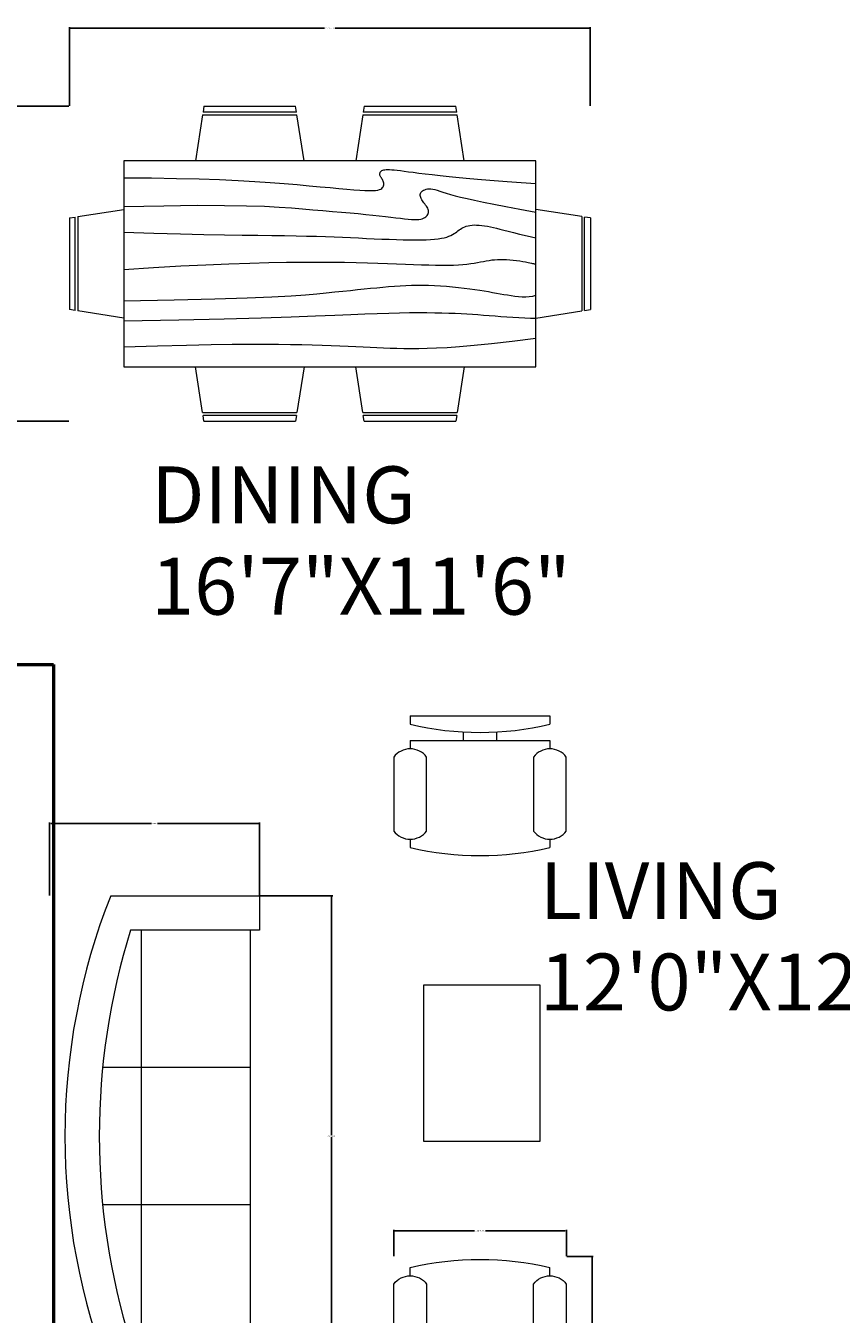
# Model space of a CAD drawing. Units: inches. Extents: x 614 to 1202, y 131 to 752.
# Tile 3 of 5: x 862 to 1005, y 293 to 518. Entities that reach past the tile are written whole.
import ezdxf

# ---------------------------------------------------------------- set-up
doc = ezdxf.new("R2010")
doc.units = ezdxf.units.IN
doc.header["$MEASUREMENT"] = 0
for name, color, linetype, lineweight in [('A-ANNO-DIMS', 2, 'Continuous', 18), ('A-AREA-IDEN', 7, 'Continuous', 18), ('A-FURN', 8, 'Continuous', 18), ('A-WALL', 7, 'Continuous', 50)]:
    doc.layers.add(name, color=color, linetype=linetype, lineweight=lineweight)
doc.styles.get("Standard").update_dxf_attribs({"font": 'arial.ttf'})
doc.dimstyles.get("Standard").update_dxf_attribs({"dimtxt": 0.18, "dimasz": 0.18, "dimexe": 0.18, "dimexo": 0.0625, "dimgap": 0.09, "dimtad": 0, "dimtih": 1, "dimtoh": 1, "dimdec": 0, "dimzin": 0, "dimdsep": 46, "dimlunit": 3, "dimtxsty": 'Standard', "dimcen": 0.09, "dimadec": 0, "dimazin": 0, "dimtfac": 1, "dimtdec": 0, "dimtofl": 0, "dimtmove": 0, "dimatfit": 3, "dimfxl": 1, "dimtolj": 1, "dimtzin": 0, "dimarcsym": 0})

# ---------------------------------------------------------------- blocks, each defined once
blk = doc.blocks.new('Sofa - Roundback 7 ft.')
for p, q in [((-12.00002, -32.4421), (-12.00003, -6.5971)), ((11.99997, -32.4421), (11.99998, -6.5971)), ((-36.000027, -34), (-36.000027, -11.4696)), ((-35.999844, -13.3819), (35.9998, -13.3819)), ((35.99998, -34), (35.99998, -11.4696)), ((-36.000027, -32.4421), (35.99998, -32.4421))]:
    blk.add_line(p, q)
for points in [[(-36.000027, -34), (-42.000027, -34), (-42.000027, -8)], [(41.99998, -8), (41.99998, -34), (35.99998, -34)]]:
    blk.add_lwpolyline(points)
for centre, radius, start, end in [((0, -114.25), 114.25, 68.43141, 111.5686), ((-0.00001, -127.1968), 121.1968, 72.72033, 107.2797)]:
    blk.add_arc(centre, radius, start, end)
blk = doc.blocks.new('Chair - Desk')
for p, q in [((-8.5, 0), (-8.5, -1)), ((-8.5, 0), (8.5, 0)), ((8.5, 0), (8.5, -1)), ((-8.5, -3), (-8.5, -4)), ((-8.5, -3), (8.5, -3)), ((-2, -3), (-2, -1.9355)), ((2, -1.9576), (2, -3)), ((8.5, -3), (8.5, -4)), ((-10.5, -5), (-10.5, -14)), ((-6.5, -14), (-6.5, -5)), ((6.5, -5), (6.5, -14)), ((10.5, -14), (10.5, -5)), ((-8.5, -15), (-8.5, -16)), ((8.5, -15), (8.5, -16))]:
    blk.add_line(p, q)
for centre, radius, start, end in [((0, 34.625), 36.625, 256.5803, 283.4197), ((-8.5, -6.5), 2.5, 36.8699, 143.1301), ((8.5, -6.5), 2.5, 36.8699, 143.1301), ((-8.5, -12.5), 2.5, 216.8699, 323.1301), ((8.5, -12.5), 2.5, 216.8699, 323.1301), ((0, 19.625), 36.625, 256.5803, 283.4197)]:
    blk.add_arc(centre, radius, start, end)
blk = doc.blocks.new('Dining Set - 36 x 72 in.')
for p, q in [((-22, 27.5), (-22.1562, 26.50042)), ((-22, 27.5), (-6, 27.5)), ((-5.8437, 26.49966), (-6, 27.5)), ((6, 27.5), (5.8438, 26.50042)), ((6, 27.5), (22, 27.5)), ((22.1563, 26.49966), (22, 27.5)), ((-22.2343, 26.00059), (-23.4847, 17.99762)), ((-22.2304, 26), (-5.7608, 26)), ((-5.8416, 26.5), (-22.1534, 26.5)), ((-4.5152, 17.99762), (-5.7655, 25.99926)), ((5.7657, 26.00059), (4.5153, 17.99762)), ((5.7696, 26), (22.2392, 26)), ((22.1584, 26.5), (5.8466, 26.5)), ((23.4848, 17.99762), (22.2345, 25.99926)), ((36, 18), (-36, 18)), ((-36, 18), (-36, -18)), ((36, -18), (36, 18)), ((-44.0006, 8.23428), (-35.9976, 9.48474)), ((44.0006, 8.23428), (35.9976, 9.48474)), ((-45.5, 8), (-44.5004, 8.15617)), ((-45.5, 8), (-45.5, -8)), ((-44.5, -8.15843), (-44.5, 8.15338)), ((-44, 8.23041), (-44, -8.23915)), ((44, 8.23041), (44, -8.23915)), ((44.5, -8.15843), (44.5, 8.15338)), ((45.5, 8), (44.5005, 8.15617)), ((45.5, 8), (45.5, -8)), ((-44.4997, -8.15631), (-45.5, -8)), ((-35.9976, -9.48476), (-43.9993, -8.2345)), ((35.9976, -9.48476), (43.9993, -8.2345)), ((44.4997, -8.15631), (45.5, -8)), ((-36, -18), (36, -18)), ((-22.2343, -26.0006), (-23.4847, -17.99762)), ((-4.5152, -17.99762), (-5.7655, -25.99928)), ((5.7657, -26.0006), (4.5153, -17.99762)), ((23.4848, -17.99762), (22.2345, -25.99928)), ((-22.2304, -26), (-5.7608, -26)), ((-22, -27.5), (-22.1562, -26.50044)), ((-5.8416, -26.5), (-22.1534, -26.5)), ((-5.8437, -26.49967), (-6, -27.5)), ((5.7696, -26), (22.2392, -26)), ((6, -27.5), (5.8438, -26.50044)), ((22.1584, -26.5), (5.8466, -26.5)), ((22.1563, -26.49967), (22, -27.5)), ((-22, -27.5), (-6, -27.5)), ((6, -27.5), (22, -27.5))]:
    blk.add_line(p, q)
for points in [[(-36, 15), (-31.1772, 14.97754), (-26.8079, 14.91406), (-22.8538, 14.81543), (-19.276, 14.6875), (-16.0362, 14.53613), (-13.0957, 14.36718), (-10.4159, 14.18652), (-7.9583, 14), (-5.6904, 13.81315), (-3.6035, 13.63021), (-1.6954, 13.45508), (0.0365, 13.29166), (1.5945, 13.14388), (2.9811, 13.01562), (4.1988, 12.9108), (5.25, 12.83333), (6.1393, 12.78613), (6.8802, 12.76823), (7.4883, 12.77767), (7.9792, 12.8125), (8.3685, 12.87077), (8.6719, 12.95052), (8.9049, 13.0498), (9.0833, 13.16666), (9.2205, 13.29899), (9.3216, 13.44401), (9.3895, 13.59879), (9.4271, 13.76041), (9.4373, 13.92594), (9.4232, 14.09245), (9.3875, 14.257), (9.3333, 14.41666), (9.2638, 14.56917), (9.1836, 14.71484), (9.0975, 14.85465), (9.0104, 14.98958), (8.9272, 15.1206), (8.8529, 15.2487), (8.7922, 15.37483), (8.75, 15.5), (8.7305, 15.62467), (8.7344, 15.74739), (8.7617, 15.86621), (8.8125, 15.97916), (8.8867, 16.08431), (8.9844, 16.17968), (9.1055, 16.26334), (9.25, 16.33333), (9.4189, 16.38802), (9.6172, 16.42708), (9.8506, 16.45052), (10.125, 16.45833), (10.4463, 16.45052), (10.8203, 16.42708), (11.2529, 16.38802), (11.75, 16.33333), (12.3184, 16.26318), (12.9694, 16.17838), (13.7151, 16.07991), (14.5677, 15.96875), (15.5395, 15.84586), (16.6426, 15.71224), (17.8893, 15.56884), (19.2917, 15.41666), (20.859, 15.25667), (22.5879, 15.08984), (24.4721, 14.91715), (26.5052, 14.73958), (28.6809, 14.5581), (30.9929, 14.3737), (33.4347, 14.18733), (36, 14)], [(-36, 10), (-28.9766, 10.14274), (-23.1725, 10.20442), (-18.4241, 10.19775), (-14.5677, 10.13541), (-11.4399, 10.03011), (-8.877, 9.89453), (-6.7154, 9.74137), (-4.7917, 9.58333), (-2.9698, 9.43082), (-1.2246, 9.28515), (0.4415, 9.14534), (2.026, 9.01041), (3.5266, 8.87939), (4.9408, 8.7513), (6.266, 8.62516), (7.5, 8.5), (8.6411, 8.37549), (9.6914, 8.2539), (10.6538, 8.13818), (11.5312, 8.03125), (12.3267, 7.93603), (13.043, 7.85547), (13.6831, 7.79248), (14.25, 7.75), (14.7471, 7.7303), (15.1797, 7.73307), (15.5537, 7.75732), (15.875, 7.80208), (16.1494, 7.86637), (16.3828, 7.94922), (16.5811, 8.04964), (16.75, 8.16666), (16.8944, 8.29915), (17.0143, 8.44531), (17.1089, 8.60319), (17.1771, 8.77083), (17.218, 8.94629), (17.2305, 9.1276), (17.2137, 9.31282), (17.1667, 9.5), (17.0895, 9.6875), (16.987, 9.875), (16.8649, 10.0625), (16.7292, 10.25), (16.5856, 10.4375), (16.4401, 10.625), (16.2985, 10.8125), (16.1667, 11), (16.05, 11.18733), (15.9518, 11.3737), (15.8752, 11.5581), (15.8229, 11.73958), (15.798, 11.91715), (15.8034, 12.08984), (15.842, 12.25667), (15.9167, 12.41666), (16.0295, 12.56836), (16.1784, 12.70833), (16.3605, 12.83268), (16.5729, 12.9375), (16.8127, 13.01888), (17.0768, 13.07291), (17.3625, 13.0957), (17.6667, 13.08333), (17.9894, 13.03312), (18.3418, 12.94726), (18.7382, 12.82918), (19.1927, 12.68229), (19.7195, 12.51001), (20.3327, 12.31575), (21.0465, 12.10294), (21.875, 11.875), (22.8357, 11.63354), (23.959, 11.37304), (25.2786, 11.08618), (26.8282, 10.76562), (28.6414, 10.40405), (30.752, 9.99414), (33.1936, 9.52856), (36, 9)], [(-36, 5.5), (-30.7157, 5.3348), (-26.069, 5.20963), (-21.9946, 5.11767), (-18.4271, 5.05208), (-15.3009, 5.00602), (-12.5508, 4.97265), (-10.1112, 4.94515), (-7.9167, 4.91666), (-5.909, 4.88167), (-4.0586, 4.83984), (-2.3429, 4.79215), (-0.7396, 4.73958), (0.7739, 4.6831), (2.22, 4.6237), (3.6213, 4.56233), (5, 4.5), (6.373, 4.43782), (7.7344, 4.3776), (9.0723, 4.32129), (10.375, 4.27083), (11.6309, 4.22819), (12.8281, 4.19531), (13.9551, 4.17415), (15, 4.16666), (15.954, 4.17448), (16.819, 4.19791), (17.6001, 4.23698), (18.3021, 4.29166), (18.9299, 4.36198), (19.4883, 4.44791), (19.9823, 4.54948), (20.4167, 4.66666), (20.7969, 4.79899), (21.1302, 4.94401), (21.4245, 5.09879), (21.6875, 5.26041), (21.9271, 5.42594), (22.1511, 5.59245), (22.3672, 5.757), (22.5834, 5.91666), (22.8065, 6.06868), (23.0404, 6.21093), (23.2879, 6.34147), (23.5521, 6.45833), (23.8358, 6.55957), (24.142, 6.64323), (24.4735, 6.70735), (24.8334, 6.75), (25.2235, 6.76969), (25.642, 6.76692), (26.0858, 6.74267), (26.5521, 6.69791), (27.0379, 6.63362), (27.5404, 6.55078), (28.0565, 6.45036), (28.5834, 6.33333), (29.1242, 6.19987), (29.7071, 6.04687), (30.3661, 5.87044), (31.1354, 5.66666), (32.0493, 5.43164), (33.142, 5.16146), (34.4475, 4.85221), (36, 4.5)], [(-36, -1), (-30.7915, -0.6591), (-26.0195, -0.38216), (-21.6519, -0.16284), (-17.6563, 0.00521), (-14.0005, 0.12833), (-10.6523, 0.21289), (-7.5796, 0.26522), (-4.75, 0.29166), (-2.134, 0.29793), (0.2878, 0.28711), (2.5317, 0.26163), (4.6146, 0.22396), (6.5529, 0.17651), (8.3633, 0.12174), (10.0623, 0.06209), (11.6667, 0), (13.1899, -0.06201), (14.6341, -0.1211), (15.9982, -0.17432), (17.2813, -0.21875), (18.4823, -0.25147), (19.6003, -0.26953), (20.6343, -0.27002), (21.5834, -0.25), (22.4481, -0.20768), (23.2357, -0.14584), (23.9549, -0.06836), (24.6146, 0.02083), (25.2235, 0.11784), (25.7904, 0.21875), (26.3241, 0.31966), (26.8334, 0.41666), (27.3265, 0.50618), (27.8099, 0.58593), (28.2894, 0.65397), (28.7709, 0.70833), (29.2601, 0.74707), (29.763, 0.76823), (30.2855, 0.76985), (30.8334, 0.75), (31.4088, 0.70784), (31.9994, 0.64713), (32.589, 0.57275), (33.1615, 0.48958), (33.7008, 0.4025), (34.1908, 0.3164), (34.6153, 0.23616), (34.9584, 0.16666), (35.2099, 0.11165), (35.3848, 0.07031), (35.504, 0.04069), (35.5886, 0.02083), (35.6594, 0.00879), (35.7377, 0.0026), (35.8442, 0.00032), (36, 0)], [(-36, -6.5), (-27.1843, -6.31267), (-20.084, -6.1263), (-14.469, -5.9419), (-10.1094, -5.76042), (-6.7752, -5.58285), (-4.2363, -5.41016), (-2.2629, -5.24333), (-0.625, -5.08334), (0.8708, -4.93099), (2.2715, -4.78646), (3.5872, -4.64974), (4.8281, -4.52084), (6.0046, -4.39974), (7.127, -4.28646), (8.2053, -4.18099), (9.25, -4.08334), (10.2705, -3.99382), (11.2734, -3.91407), (12.2647, -3.84603), (13.25, -3.79167), (14.2354, -3.75293), (15.2266, -3.73177), (16.2295, -3.73015), (17.25, -3.75), (18.2912, -3.79248), (19.3451, -3.85547), (20.4009, -3.93604), (21.4479, -4.03125), (22.4754, -4.13819), (23.4727, -4.25391), (24.4289, -4.37549), (25.3334, -4.5), (26.1785, -4.62492), (26.9694, -4.74935), (27.7145, -4.87281), (28.4219, -4.99479), (29.1, -5.11483), (29.7572, -5.23242), (30.4016, -5.34709), (31.0417, -5.45834), (31.6837, -5.56437), (32.3262, -5.65821), (32.9658, -5.73153), (33.599, -5.77604), (34.2224, -5.78345), (34.8327, -5.74545), (35.4264, -5.65373), (36, -5.5)], [(-36, -10), (-26.4022, -9.81299), (-18.4675, -9.62891), (-11.9839, -9.45069), (-6.7396, -9.28125), (-2.5226, -9.12354), (0.8789, -8.98047), (3.6769, -8.85498), (6.0833, -8.75), (8.2767, -8.66765), (10.3021, -8.60677), (12.1712, -8.56543), (13.8958, -8.54167), (15.4876, -8.53353), (16.9583, -8.53907), (18.3197, -8.55632), (19.5834, -8.58334), (20.7616, -8.61841), (21.8685, -8.66081), (22.9188, -8.71004), (23.9271, -8.76563), (24.9081, -8.82707), (25.8763, -8.89388), (26.8465, -8.96558), (27.8334, -9.04167), (28.8474, -9.12118), (29.8828, -9.20117), (30.93, -9.27824), (31.9792, -9.34896), (33.0205, -9.40991), (34.0443, -9.45768), (35.0407, -9.48885), (36, -9.5)], [(-36, -14.5), (-30.0881, -14.33513), (-25.0332, -14.21224), (-20.7312, -14.12647), (-17.0781, -14.07292), (-13.97, -14.04671), (-11.3027, -14.04297), (-8.9724, -14.05681), (-6.875, -14.08334), (-4.9224, -14.11833), (-3.0905, -14.16016), (-1.3709, -14.20785), (0.2448, -14.26042), (1.7647, -14.3169), (3.1973, -14.3763), (4.5507, -14.43767), (5.8333, -14.5), (7.0554, -14.5621), (8.235, -14.62175), (9.3922, -14.67652), (10.5469, -14.72396), (11.7192, -14.76164), (12.929, -14.78711), (14.1965, -14.79794), (15.5417, -14.79167), (16.9933, -14.76424), (18.6152, -14.70508), (20.4804, -14.60197), (22.6615, -14.44271), (25.2312, -14.21509), (28.2624, -13.9069), (31.8277, -13.50594), (36, -13)]]:
    blk.add_lwpolyline(points)
blk = doc.blocks.new('*D13')
at = {"layer": 'A-ANNO-DIMS', "color": 0, "lineweight": -2, "transparency": 16777216}
for p, q in [((926.44, 302.89), (926.44, 307.53)), ((926.62, 307.35), (940.55, 307.35)), ((956.4, 307.35), (942.46, 307.35)), ((956.58, 302.89), (956.58, 307.53))]:
    blk.add_line(p, q, dxfattribs=at)
at = {"layer": 'A-ANNO-DIMS', "color": 0, "transparency": 16777216}
for points in [[(926.62, 307.38), (926.62, 307.32), (926.44, 307.35)], [(956.4, 307.38), (956.4, 307.32), (956.58, 307.35)]]:
    blk.add_solid(points, dxfattribs=at)
at = {"layer": 'Defpoints', "color": 0, "transparency": 16777216}
for p in [(956.58, 307.35), (926.44, 302.83), (956.58, 302.83)]:
    blk.add_point(p, dxfattribs=at)
at = {"layer": 'A-ANNO-DIMS', "color": 0, "transparency": 16777216, "insert": (941.51, 307.35), "char_height": 0.18, "attachment_point": 5}
blk.add_mtext('\\A1;CHAIR 30 TYP.', dxfattribs=at)
blk = doc.blocks.new('*D14')
at = {"layer": 'A-ANNO-DIMS', "color": 0, "lineweight": -2, "transparency": 16777216}
for p, q in [((956.64, 302.83), (961.28, 302.83)), ((961.1, 302.65), (961.1, 290.57)), ((961.1, 278.13), (961.1, 290.21)), ((956.64, 277.95), (961.28, 277.95))]:
    blk.add_line(p, q, dxfattribs=at)
at = {"layer": 'A-ANNO-DIMS', "color": 0, "transparency": 16777216}
for points in [[(961.07, 302.65), (961.13, 302.65), (961.1, 302.83)], [(961.07, 278.13), (961.13, 278.13), (961.1, 277.95)]]:
    blk.add_solid(points, dxfattribs=at)
at = {"layer": 'Defpoints', "color": 0, "transparency": 16777216}
for p in [(956.58, 302.83), (956.58, 277.95), (961.1, 277.95)]:
    blk.add_point(p, dxfattribs=at)
at = {"layer": 'A-ANNO-DIMS', "color": 0, "transparency": 16777216, "insert": (961.1, 290.39), "char_height": 0.18, "attachment_point": 5}
blk.add_mtext('\\A1;25 TYP.', dxfattribs=at)
blk = doc.blocks.new('*D27')
at = {"layer": 'A-ANNO-DIMS', "color": 0, "lineweight": -2, "transparency": 16777216}
for p, q in [((903.06, 365.86), (915.77, 365.86)), ((915.59, 365.68), (915.59, 324.04)), ((915.59, 282.04), (915.59, 323.68)), ((903.06, 281.86), (915.77, 281.86))]:
    blk.add_line(p, q, dxfattribs=at)
at = {"layer": 'A-ANNO-DIMS', "color": 0, "transparency": 16777216}
for points in [[(915.56, 365.68), (915.62, 365.68), (915.59, 365.86)], [(915.56, 282.04), (915.62, 282.04), (915.59, 281.86)]]:
    blk.add_solid(points, dxfattribs=at)
at = {"layer": 'Defpoints', "color": 0, "transparency": 16777216}
for p in [(902.99, 365.86), (915.59, 365.86), (902.99, 281.86)]:
    blk.add_point(p, dxfattribs=at)
at = {"layer": 'A-ANNO-DIMS', "color": 0, "transparency": 16777216, "insert": (915.59, 323.86), "char_height": 0.18, "attachment_point": 5}
blk.add_mtext('\\A1;SOFA 84 TYP.', dxfattribs=at)
blk = doc.blocks.new('*D28')
at = {"layer": 'A-ANNO-DIMS', "color": 0, "lineweight": -2, "transparency": 16777216}
for p, q in [((866.33, 365.92), (866.33, 378.64)), ((866.51, 378.46), (884.13, 378.46)), ((902.81, 378.46), (885.19, 378.46)), ((902.99, 365.92), (902.99, 378.64))]:
    blk.add_line(p, q, dxfattribs=at)
at = {"layer": 'A-ANNO-DIMS', "color": 0, "transparency": 16777216}
for points in [[(866.51, 378.49), (866.51, 378.43), (866.33, 378.46)], [(902.81, 378.49), (902.81, 378.43), (902.99, 378.46)]]:
    blk.add_solid(points, dxfattribs=at)
at = {"layer": 'Defpoints', "color": 0, "transparency": 16777216}
for p in [(866.33, 378.46), (866.33, 365.86), (902.99, 365.86)]:
    blk.add_point(p, dxfattribs=at)
at = {"layer": 'A-ANNO-DIMS', "color": 0, "transparency": 16777216, "insert": (884.66, 378.46), "char_height": 0.18, "attachment_point": 5}
blk.add_mtext('\\A1;37 TYP.', dxfattribs=at)
blk = doc.blocks.new('*D33')
at = {"layer": 'A-ANNO-DIMS', "color": 0, "lineweight": -2, "transparency": 16777216}
for p, q in [((869.77, 503.82), (869.77, 517.59)), ((869.95, 517.41), (914.32, 517.41)), ((960.59, 517.41), (916.23, 517.41)), ((960.77, 503.82), (960.77, 517.59))]:
    blk.add_line(p, q, dxfattribs=at)
at = {"layer": 'A-ANNO-DIMS', "color": 0, "transparency": 16777216}
for points in [[(869.95, 517.44), (869.95, 517.38), (869.77, 517.41)], [(960.59, 517.44), (960.59, 517.38), (960.77, 517.41)]]:
    blk.add_solid(points, dxfattribs=at)
at = {"layer": 'Defpoints', "color": 0, "transparency": 16777216}
for p in [(960.77, 517.41), (869.77, 503.76), (960.77, 503.76)]:
    blk.add_point(p, dxfattribs=at)
at = {"layer": 'A-ANNO-DIMS', "color": 0, "transparency": 16777216, "insert": (915.27, 517.41), "char_height": 0.18, "attachment_point": 5}
blk.add_mtext('\\A1;DINING SET 91', dxfattribs=at)
blk = doc.blocks.new('*D34')
at = {"layer": 'A-ANNO-DIMS', "color": 0, "lineweight": -2, "transparency": 16777216}
for p, q in [((869.71, 503.76), (855.94, 503.76)), ((856.12, 503.58), (856.12, 476.44)), ((856.12, 448.94), (856.12, 476.08)), ((869.71, 448.76), (855.94, 448.76))]:
    blk.add_line(p, q, dxfattribs=at)
at = {"layer": 'A-ANNO-DIMS', "color": 0, "transparency": 16777216}
for points in [[(856.09, 503.58), (856.15, 503.58), (856.12, 503.76)], [(856.09, 448.94), (856.15, 448.94), (856.12, 448.76)]]:
    blk.add_solid(points, dxfattribs=at)
at = {"layer": 'Defpoints', "color": 0, "transparency": 16777216}
for p in [(856.12, 503.76), (869.77, 503.76), (869.77, 448.76)]:
    blk.add_point(p, dxfattribs=at)
at = {"layer": 'A-ANNO-DIMS', "color": 0, "transparency": 16777216, "insert": (856.12, 476.26), "char_height": 0.18, "attachment_point": 5}
blk.add_mtext('\\A1;55', dxfattribs=at)

msp = doc.modelspace()

# ---------------------------------------------------------------- linework, layer by layer
at = {"layer": 'A-FURN'}
msp.add_lwpolyline([(931.7159, 350.321), (951.9517, 350.321), (951.9517, 322.9369), (931.7159, 322.9369)], close=True, dxfattribs=at)
at = {"layer": 'A-WALL'}
for p, q in [((856.9938, 406.2636), (866.9938, 406.2636)), ((866.9938, 406.2636), (866.9938, 264.2636))]:
    msp.add_line(p, q, dxfattribs=at)

# ---------------------------------------------------------------- block references
at = {"layer": 'A-FURN'}
msp.add_blockref('Dining Set - 36 x 72 in.', (915.2738, 476.2604), dxfattribs=at)
at = {"layer": 'A-FURN', "xscale": 1.435269817045705, "yscale": 1.435269817045705, "zscale": 1.435269817045705}
msp.add_blockref('Chair - Desk', (941.5074, 397.2651), dxfattribs=at)
at = {"layer": 'A-FURN', "rotation": 90}
msp.add_blockref('Sofa - Roundback 7 ft.', (868.9942, 323.8607), dxfattribs=at)
at = {"layer": 'A-FURN', "xscale": -1.435269817045705, "yscale": 1.435269817045705, "zscale": 1.435269817045705, "rotation": 180}
msp.add_blockref('Chair - Desk', (941.5074, 277.9487), dxfattribs=at)

# ---------------------------------------------------------------- texts
at = {"layer": 'A-AREA-IDEN'}
for s, p in [('DINING', (884.0544, 430.9234)), ('16\'7"X11\'6"', (884.0544, 414.9609)), ('LIVING', (951.9517, 361.7904)), ('12\'0"X12\'7"', (951.9517, 345.8279))]:
    msp.add_text(s, height=9.93672, dxfattribs=at).set_placement(p)

# ---------------------------------------------------------------- dimensions: what is measured, and where the dimension line sits
at = {"layer": 'A-ANNO-DIMS'}
for base, p1, p2, text, picture, middle in [((960.7738, 517.4104), (869.7738, 503.7604), (960.7738, 503.7604), 'DINING SET <>', '*D33', (915.2738, 517.4104)), ((956.5778, 307.3478), (926.4371, 302.8267), (956.5778, 302.8267), 'CHAIR <> TYP.', '*D13', (941.5074, 307.3478))]:
    dim = msp.add_linear_dim(base=base, p1=p1, p2=p2, text=text, dimstyle='Standard', override={"dimdec": 0, "dimlfac": 1, "dimrnd": 0, "dimzin": 0, "dimdsep": 46, "dimlunit": 2}, dxfattribs=at)
    dim.commit()
    dim.dimension.update_dxf_attribs({"geometry": picture, "text_midpoint": middle})
dim = msp.add_linear_dim(base=(856.1238, 503.7604), p1=(869.7738, 448.7604), p2=(869.7738, 503.7604), angle=90, dimstyle='Standard', override={"dimdec": 0, "dimlfac": 1, "dimrnd": 0, "dimzin": 0, "dimdsep": 46, "dimlunit": 2}, dxfattribs=at)
dim.commit()
dim.dimension.update_dxf_attribs({"geometry": '*D34', "text_midpoint": (856.1238, 476.2604)})
for base, p1, p2, angle, text, picture, middle in [((866.3276, 378.4607), (902.9942, 365.8607), (866.3276, 365.8607), 180, '<> TYP.', '*D28', (884.6609, 378.4607)), ((915.5942, 365.8607), (902.9942, 281.8607), (902.9942, 365.8607), 90, 'SOFA <> TYP.', '*D27', (915.5942, 323.8607)), ((961.0989, 277.9487), (956.5778, 302.8267), (956.5778, 277.9487), 270, '<> TYP.', '*D14', (961.0989, 290.3877))]:
    dim = msp.add_linear_dim(base=base, p1=p1, p2=p2, angle=angle, text=text, dimstyle='Standard', override={"dimdec": 0, "dimlfac": 1, "dimrnd": 0, "dimzin": 0, "dimdsep": 46, "dimlunit": 2}, dxfattribs=at)
    dim.commit()
    dim.dimension.update_dxf_attribs({"geometry": picture, "text_midpoint": middle})

doc.saveas('drawing.dxf')
